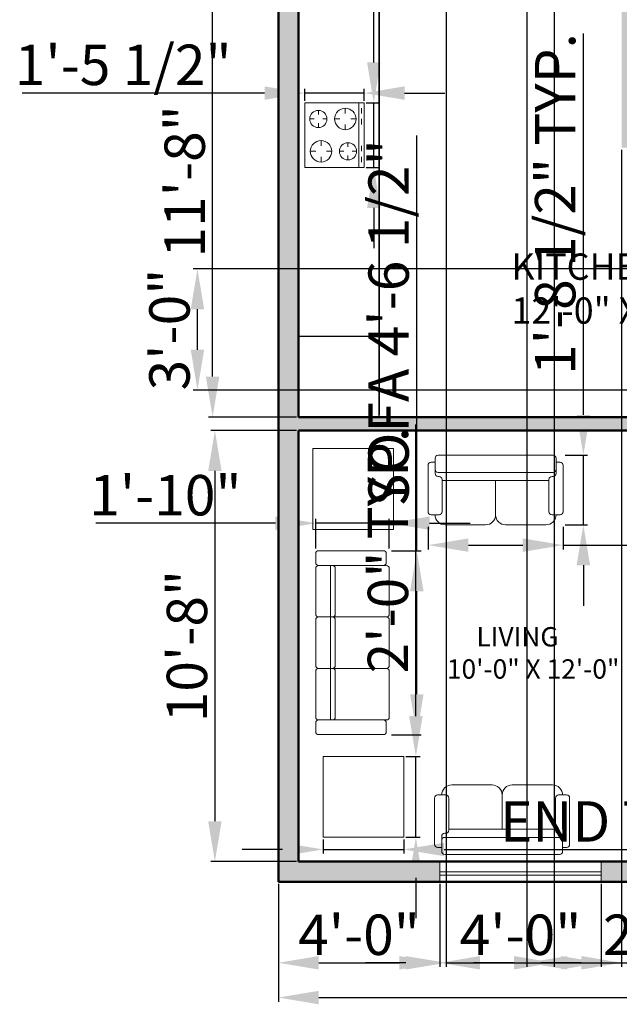
# Model space of a CAD drawing. Units: inches. Extents: x 2549 to 2991, y 1646 to 2183.
# Tile 1 of 3: x 2549 to 2727, y 1646 to 1938. Entities that reach past the tile are written whole.
import ezdxf

# ---------------------------------------------------------------- set-up
doc = ezdxf.new("R2010")
doc.units = ezdxf.units.IN
for name, color, linetype, lineweight in [('A-ANNO-DIMS', 2, 'Continuous', 18), ('A-AREA-IDEN', 7, 'Continuous', 25), ('A-EQPM', 8, 'Continuous', 20), ('A-FLOR-CASE', 8, 'Continuous', 25), ('A-FURN', 9, 'Continuous', 18), ('A-GLAZ', 4, 'Continuous', 18), ('A-WALL', 7, 'Continuous', 50)]:
    doc.layers.add(name, color=color, linetype=linetype, lineweight=lineweight)
doc.layers.add('A-WALL-PATT', color=251, linetype='Continuous', lineweight=13, true_color=0x636466)
doc.styles.get("Standard").update_dxf_attribs({"font": 'arial.ttf'})
doc.dimstyles.new('ISO-25', dxfattribs={"dimtxt": 12, "dimasz": 12, "dimexe": 1.25, "dimexo": 0.625, "dimtad": 1, "dimlunit": 3, "dimtxsty": 'Standard', "dimcen": 2.5, "dimadec": 0, "dimazin": 0, "dimtfac": 1, "dimtmove": 0, "dimatfit": 3, "dimfxl": 1, "dimarcsym": 0})

# ---------------------------------------------------------------- blocks, each defined once
blk = doc.blocks.new('A$C02A636C4')
for p, q in [((1.2026, 0.6692), (0.097, 0.6692)), ((0, 0.5722), (0, 0.1261)), ((0.0679, 0.6013), (0.0291, 0.6013)), ((0.0679, 0.6401), (0.0679, 0.6013)), ((0.0679, 0.5334), (0.0679, 0.6013)), ((1.2317, 0.6401), (1.2317, 0.6013)), ((1.2317, 0.6013), (1.2705, 0.6013)), ((1.2317, 0.5334), (1.2317, 0.6013)), ((1.2996, 0.5722), (1.2996, 0.1261)), ((0.0679, 0.4946), (0.0679, 0.5431)), ((1.2026, 0.5043), (0.097, 0.5043)), ((1.2317, 0.4946), (1.2317, 0.5431)), ((0.1067, 0.4655), (0.097, 0.4655)), ((0.1358, 0.1261), (0.1358, 0.4364)), ((1.1638, 0.4267), (0.1358, 0.4267)), ((0.6498, 0.097), (0.6498, 0.4267)), ((1.1638, 0.1261), (1.1638, 0.4364)), ((1.1929, 0.4655), (1.2026, 0.4655)), ((0.0291, 0.097), (0.1067, 0.097)), ((1.2705, 0.097), (1.1929, 0.097)), ((0.1649, 0), (0.5528, 0)), ((0.7468, 0), (1.1347, 0))]:
    blk.add_line(p, q)
for centre, radius, start, end in [((0.097, 0.6401), 0.0291, 90, 180), ((1.2026, 0.6401), 0.0291, 0, 90), ((0.0291, 0.5722), 0.0291, 90, 180), ((1.2705, 0.5722), 0.0291, 0, 90), ((0.097, 0.5334), 0.0291, 180, 270), ((0.097, 0.4946), 0.0291, 180, 270), ((1.2026, 0.5334), 0.0291, 270, 0), ((1.2026, 0.4946), 0.0291, 270, 0), ((0.1067, 0.4364), 0.0291, 0, 90), ((1.1929, 0.4364), 0.0291, 90, 180), ((0.0291, 0.1261), 0.0291, 180, 270), ((0.1649, 0.097), 0.097, 180, 270), ((0.1067, 0.1261), 0.0291, 270, 0), ((0.5528, 0.097), 0.097, 270, 0), ((0.7468, 0.097), 0.097, 180, 270), ((1.1347, 0.097), 0.097, 270, 0), ((1.1929, 0.1261), 0.0291, 180, 270), ((1.2705, 0.1261), 0.0291, 270, 0)]:
    blk.add_arc(centre, radius, start, end)
blk = doc.blocks.new('A$C0513100E')
for p, q in [((0, 0.768), (0, 0.064)), ((0.032, 0.8), (0.128, 0.8)), ((0.16, 0.768), (0.16, 0.032)), ((0.688, 0.8), (0.192, 0.8)), ((0.72, 0.768), (0.72, 0.032)), ((1.248, 0.8), (0.752, 0.8)), ((1.28, 0.768), (1.28, 0.032)), ((1.808, 0.8), (1.312, 0.8)), ((1.84, 0.032), (1.84, 0.768)), ((1.872, 0.8), (1.968, 0.8)), ((2, 0.064), (2, 0.768)), ((0.72, 0.64), (0.16, 0.64)), ((0.688, 0.587), (0.192, 0.587)), ((1.28, 0.64), (0.72, 0.64)), ((1.248, 0.587), (0.752, 0.587)), ((1.84, 0.64), (1.28, 0.64)), ((1.808, 0.587), (1.312, 0.587)), ((0.72, 0.064), (0.72, 0.402)), ((1.28, 0.064), (1.28, 0.402)), ((1.84, 0.064), (1.84, 0.402)), ((0.032, 0.032), (0.128, 0.032)), ((0.192, 0), (0.688, 0)), ((0.752, 0), (1.248, 0)), ((1.312, 0), (1.808, 0)), ((1.872, 0.032), (1.968, 0.032))]:
    blk.add_line(p, q)
for centre, start, end in [((0.032, 0.768), 90, 180), ((0.128, 0.768), 0, 90), ((0.192, 0.768), 90, 180), ((0.688, 0.768), 0, 90), ((0.752, 0.768), 90, 180), ((1.248, 0.768), 0, 90), ((1.312, 0.768), 90, 180), ((1.808, 0.768), 0, 90), ((1.872, 0.768), 90, 180), ((1.968, 0.768), 0, 90), ((0.192, 0.619), 180, 270), ((0.688, 0.619), 270, 0), ((0.752, 0.619), 180, 270), ((1.248, 0.619), 270, 0), ((1.312, 0.619), 180, 270), ((1.808, 0.619), 270, 0), ((0.032, 0.064), 180, 270), ((0.128, 0.064), 270, 0), ((0.192, 0.032), 180, 270), ((0.688, 0.032), 270, 0), ((0.752, 0.032), 180, 270), ((1.248, 0.032), 270, 0), ((1.312, 0.032), 180, 270), ((1.808, 0.032), 270, 0), ((1.872, 0.064), 180, 270), ((1.968, 0.064), 270, 0)]:
    blk.add_arc(centre, 0.032, start, end)
blk = doc.blocks.new('A$C3FB84F07')
at = {"linetype": 'ByBlock'}
for p, q in [((487.7, 447), (0, 447)), ((0, 447), (0, 0)), ((487.7, 0), (487.7, 447)), ((121.9, 406.4), (121.9, 365.8)), ((365.8, 410.5), (365.8, 378)), ((40.6, 325.1), (81.3, 325.1)), ((203.2, 325.1), (162.6, 325.1)), ((300.7, 345.4), (333.2, 345.4)), ((365.8, 280.4), (365.8, 312.9)), ((430.8, 345.4), (398.3, 345.4)), ((121.9, 243.8), (121.9, 284.5)), ((365.8, 223.5), (365.8, 182.9)), ((121.9, 186.9), (121.9, 154.4)), ((56.9, 121.9), (89.4, 121.9)), ((121.9, 56.9), (121.9, 89.4)), ((186.9, 121.9), (154.4, 121.9)), ((284.5, 142.2), (325.1, 142.2)), ((365.8, 61), (365.8, 101.6)), ((447, 142.2), (406.4, 142.2)), ((0, 40.6), (487.7, 40.6)), ((0, 0), (487.7, 0)), ((40.6, 20.3), (81.3, 20.3)), ((121.9, 20.3), (162.6, 20.3)), ((325.1, 20.3), (365.8, 20.3)), ((406.4, 20.3), (447, 20.3))]:
    blk.add_line(p, q, dxfattribs=at)
for centre, radius in [((121.9, 325.1), 81.3), ((365.8, 345.4), 65), ((365.8, 142.2), 81.3), ((121.9, 121.9), 65)]:
    blk.add_circle(centre, radius, dxfattribs=at)
blk = doc.blocks.new('*D11')
at = {"layer": 'A-ANNO-DIMS', "color": 0, "lineweight": -2, "transparency": 16777216}
for p, q in [((2631.41, 1960.26), (2605.25, 1960.26)), ((2606.5, 1832.26), (2606.5, 1948.26)), ((2631.41, 1820.26), (2605.25, 1820.26))]:
    blk.add_line(p, q, dxfattribs=at)
at = {"layer": 'A-ANNO-DIMS', "color": 0, "transparency": 16777216}
for points in [[(2604.5, 1948.26), (2608.5, 1948.26), (2606.5, 1960.26)], [(2604.5, 1832.26), (2608.5, 1832.26), (2606.5, 1820.26)]]:
    blk.add_solid(points, dxfattribs=at)
at = {"layer": 'Defpoints', "color": 0, "transparency": 16777216}
for p in [(2606.5, 1960.26), (2632.04, 1960.26), (2632.04, 1820.26)]:
    blk.add_point(p, dxfattribs=at)
at = {"layer": 'A-ANNO-DIMS', "color": 0, "transparency": 16777216, "insert": (2599.75, 1890.26), "char_height": 12, "attachment_point": 5, "rotation": 90}
blk.add_mtext('11\'-8"', dxfattribs=at)
blk = doc.blocks.new('*D12')
at = {"layer": 'A-ANNO-DIMS', "color": 0, "lineweight": -2, "transparency": 16777216}
for p, q in [((2631.41, 1816.26), (2605.92, 1816.26)), ((2607.17, 1804.26), (2607.17, 1700.26)), ((2631.41, 1688.26), (2605.92, 1688.26))]:
    blk.add_line(p, q, dxfattribs=at)
at = {"layer": 'A-ANNO-DIMS', "color": 0, "transparency": 16777216}
for points in [[(2605.17, 1804.26), (2609.17, 1804.26), (2607.17, 1816.26)], [(2605.17, 1700.26), (2609.17, 1700.26), (2607.17, 1688.26)]]:
    blk.add_solid(points, dxfattribs=at)
at = {"layer": 'Defpoints', "color": 0, "transparency": 16777216}
for p in [(2632.04, 1816.26), (2607.17, 1688.26), (2632.04, 1688.26)]:
    blk.add_point(p, dxfattribs=at)
at = {"layer": 'A-ANNO-DIMS', "color": 0, "transparency": 16777216, "insert": (2600.42, 1752.26), "char_height": 12, "attachment_point": 5, "rotation": 90}
blk.add_mtext('10\'-8"', dxfattribs=at)
blk = doc.blocks.new('*D13')
at = {"layer": 'A-ANNO-DIMS', "color": 0, "lineweight": -2, "transparency": 16777216}
for p, q in [((2626.04, 1681.64), (2626.04, 1646.63)), ((2866.04, 1681.64), (2866.04, 1646.63)), ((2638.04, 1647.88), (2854.04, 1647.88))]:
    blk.add_line(p, q, dxfattribs=at)
at = {"layer": 'A-ANNO-DIMS', "color": 0, "transparency": 16777216}
for points in [[(2638.04, 1649.88), (2638.04, 1645.88), (2626.04, 1647.88)], [(2854.04, 1649.88), (2854.04, 1645.88), (2866.04, 1647.88)]]:
    blk.add_solid(points, dxfattribs=at)
at = {"layer": 'Defpoints', "color": 0, "transparency": 16777216}
for p in [(2626.04, 1682.26), (2866.04, 1682.26), (2866.04, 1647.88)]:
    blk.add_point(p, dxfattribs=at)
at = {"layer": 'A-ANNO-DIMS', "color": 0, "transparency": 16777216, "insert": (2746.04, 1654.63), "char_height": 12, "attachment_point": 5}
blk.add_mtext("20'", dxfattribs=at)
blk = doc.blocks.new('END-TABLE-24')
for p, q in [((0, 24), (24, 24)), ((0, 0), (0, 24)), ((24, 24), (24, 0)), ((24, 0), (0, 0))]:
    blk.add_line(p, q)
blk = doc.blocks.new('*D16')
at = {"layer": 'A-ANNO-DIMS', "color": 0, "lineweight": -2, "transparency": 16777216}
for p, q in [((2670.52, 1787.63), (2670.52, 1780.98)), ((2710.65, 1787.63), (2710.65, 1780.98)), ((2682.52, 1782.23), (2698.65, 1782.23)), ((2710.65, 1782.23), (2889.68, 1782.23))]:
    blk.add_line(p, q, dxfattribs=at)
at = {"layer": 'A-ANNO-DIMS', "color": 0, "transparency": 16777216}
for points in [[(2682.52, 1784.23), (2682.52, 1780.23), (2670.52, 1782.23)], [(2698.65, 1784.23), (2698.65, 1780.23), (2710.65, 1782.23)]]:
    blk.add_solid(points, dxfattribs=at)
at = {"layer": 'Defpoints', "color": 0, "transparency": 16777216}
for p in [(2670.52, 1788.25), (2710.65, 1788.25), (2710.65, 1782.23)]:
    blk.add_point(p, dxfattribs=at)
at = {"layer": 'A-ANNO-DIMS', "color": 0, "transparency": 16777216, "insert": (2806.17, 1789.07), "char_height": 12, "attachment_point": 5}
blk.add_mtext('LOVESEAT 3\'-4" TYP.', dxfattribs=at)
blk = doc.blocks.new('*D17')
at = {"layer": 'A-ANNO-DIMS', "color": 0, "lineweight": -2, "transparency": 16777216}
for p, q in [((2716.67, 1820.92), (2716.67, 1934.15)), ((2711.28, 1808.92), (2717.92, 1808.92)), ((2716.67, 1788.25), (2716.67, 1808.92)), ((2711.28, 1788.25), (2717.92, 1788.25)), ((2716.67, 1776.25), (2716.67, 1764.25))]:
    blk.add_line(p, q, dxfattribs=at)
at = {"layer": 'A-ANNO-DIMS', "color": 0, "transparency": 16777216}
for points in [[(2714.67, 1820.92), (2718.67, 1820.92), (2716.67, 1808.92)], [(2714.67, 1776.25), (2718.67, 1776.25), (2716.67, 1788.25)]]:
    blk.add_solid(points, dxfattribs=at)
at = {"layer": 'Defpoints', "color": 0, "transparency": 16777216}
for p in [(2710.65, 1808.92), (2716.67, 1808.92), (2710.65, 1788.25)]:
    blk.add_point(p, dxfattribs=at)
at = {"layer": 'A-ANNO-DIMS', "color": 0, "transparency": 16777216, "insert": (2709.84, 1883.53), "char_height": 12, "attachment_point": 5, "rotation": 90}
blk.add_mtext('1\'-8 1/2" TYP.', dxfattribs=at)
blk = doc.blocks.new('*D18')
at = {"layer": 'A-ANNO-DIMS', "color": 0, "lineweight": -2, "transparency": 16777216}
for p, q in [((2639.3, 1694.84), (2639.3, 1690.62)), ((2663.3, 1694.84), (2663.3, 1690.62)), ((2627.3, 1691.87), (2615.3, 1691.87)), ((2639.3, 1691.87), (2663.3, 1691.87)), ((2675.3, 1691.87), (2858.88, 1691.87))]:
    blk.add_line(p, q, dxfattribs=at)
at = {"layer": 'A-ANNO-DIMS', "color": 0, "transparency": 16777216}
for points in [[(2627.3, 1693.87), (2627.3, 1689.87), (2639.3, 1691.87)], [(2675.3, 1693.87), (2675.3, 1689.87), (2663.3, 1691.87)]]:
    blk.add_solid(points, dxfattribs=at)
at = {"layer": 'Defpoints', "color": 0, "transparency": 16777216}
for p in [(2639.3, 1695.47), (2663.3, 1695.47), (2663.3, 1691.87)]:
    blk.add_point(p, dxfattribs=at)
at = {"layer": 'A-ANNO-DIMS', "color": 0, "transparency": 16777216, "insert": (2773.09, 1698.62), "char_height": 12, "attachment_point": 5}
blk.add_mtext('END TABLE 2\'-0" TYP.', dxfattribs=at)
blk = doc.blocks.new('*D19')
at = {"layer": 'A-ANNO-DIMS', "color": 0, "lineweight": -2, "transparency": 16777216}
for p, q in [((2666.9, 1731.47), (2666.9, 1818.07)), ((2663.93, 1719.47), (2668.15, 1719.47)), ((2666.9, 1695.47), (2666.9, 1719.47)), ((2663.93, 1695.47), (2668.15, 1695.47)), ((2666.9, 1683.47), (2666.9, 1671.47))]:
    blk.add_line(p, q, dxfattribs=at)
at = {"layer": 'A-ANNO-DIMS', "color": 0, "transparency": 16777216}
for points in [[(2664.9, 1731.47), (2668.9, 1731.47), (2666.9, 1719.47)], [(2664.9, 1683.47), (2668.9, 1683.47), (2666.9, 1695.47)]]:
    blk.add_solid(points, dxfattribs=at)
at = {"layer": 'Defpoints', "color": 0, "transparency": 16777216}
for p in [(2663.3, 1719.47), (2666.9, 1719.47), (2663.3, 1695.47)]:
    blk.add_point(p, dxfattribs=at)
at = {"layer": 'A-ANNO-DIMS', "color": 0, "transparency": 16777216, "insert": (2660.15, 1780.77), "char_height": 12, "attachment_point": 5, "rotation": 90}
blk.add_mtext('2\'-0" TYP.', dxfattribs=at)
blk = doc.blocks.new('*D22')
at = {"layer": 'A-ANNO-DIMS', "color": 0, "lineweight": -2, "transparency": 16777216}
for p, q in [((2667.18, 1780.56), (2667.18, 1903.91)), ((2659.61, 1780.56), (2668.43, 1780.56)), ((2667.18, 1737.95), (2667.18, 1768.56)), ((2659.61, 1725.95), (2668.43, 1725.95))]:
    blk.add_line(p, q, dxfattribs=at)
at = {"layer": 'A-ANNO-DIMS', "color": 0, "transparency": 16777216}
for points in [[(2665.18, 1768.56), (2669.18, 1768.56), (2667.18, 1780.56)], [(2665.18, 1737.95), (2669.18, 1737.95), (2667.18, 1725.95)]]:
    blk.add_solid(points, dxfattribs=at)
at = {"layer": 'Defpoints', "color": 0, "transparency": 16777216}
for p in [(2658.99, 1780.56), (2667.18, 1780.56), (2658.99, 1725.95)]:
    blk.add_point(p, dxfattribs=at)
at = {"layer": 'A-ANNO-DIMS', "color": 0, "transparency": 16777216, "insert": (2660.35, 1848.24), "char_height": 12, "attachment_point": 5, "rotation": 90}
blk.add_mtext('SOFA 4\'-6 1/2"', dxfattribs=at)
blk = doc.blocks.new('*D23')
at = {"layer": 'A-ANNO-DIMS', "color": 0, "lineweight": -2, "transparency": 16777216}
for p, q in [((2637.15, 1781.19), (2637.15, 1790)), ((2658.99, 1781.19), (2658.99, 1790)), ((2625.15, 1788.75), (2571.8, 1788.75)), ((2658.99, 1788.75), (2637.15, 1788.75)), ((2670.99, 1788.75), (2682.99, 1788.75))]:
    blk.add_line(p, q, dxfattribs=at)
at = {"layer": 'A-ANNO-DIMS', "color": 0, "transparency": 16777216}
for points in [[(2625.15, 1790.75), (2625.15, 1786.75), (2637.15, 1788.75)], [(2670.99, 1790.75), (2670.99, 1786.75), (2658.99, 1788.75)]]:
    blk.add_solid(points, dxfattribs=at)
at = {"layer": 'Defpoints', "color": 0, "transparency": 16777216}
for p in [(2637.15, 1788.75), (2637.15, 1780.56), (2658.99, 1780.56)]:
    blk.add_point(p, dxfattribs=at)
at = {"layer": 'A-ANNO-DIMS', "color": 0, "transparency": 16777216, "insert": (2592.47, 1795.5), "char_height": 12, "attachment_point": 5}
blk.add_mtext('1\'-10"', dxfattribs=at)
blk = doc.blocks.new('*D24')
at = {"layer": 'A-ANNO-DIMS', "color": 0, "lineweight": -2, "transparency": 16777216}
for p, q in [((2654.4, 1925.59), (2654.4, 2059.08)), ((2652.15, 1913.59), (2655.65, 1913.59)), ((2654.4, 1894.39), (2654.4, 1913.59)), ((2652.15, 1894.39), (2655.65, 1894.39)), ((2654.4, 1882.39), (2654.4, 1870.39))]:
    blk.add_line(p, q, dxfattribs=at)
at = {"layer": 'A-ANNO-DIMS', "color": 0, "transparency": 16777216}
for points in [[(2652.4, 1925.59), (2656.4, 1925.59), (2654.4, 1913.59)], [(2652.4, 1882.39), (2656.4, 1882.39), (2654.4, 1894.39)]]:
    blk.add_solid(points, dxfattribs=at)
at = {"layer": 'Defpoints', "color": 0, "transparency": 16777216}
for p in [(2651.52, 1913.59), (2654.4, 1913.59), (2651.52, 1894.39)]:
    blk.add_point(p, dxfattribs=at)
at = {"layer": 'A-ANNO-DIMS', "color": 0, "transparency": 16777216, "insert": (2647.57, 1998.33), "char_height": 12, "attachment_point": 5, "rotation": 90}
blk.add_mtext('COOKTOP 1\'-7"', dxfattribs=at)
blk = doc.blocks.new('*D25')
at = {"layer": 'A-ANNO-DIMS', "color": 0, "lineweight": -2, "transparency": 16777216}
for p, q in [((2621.92, 1916.47), (2549.94, 1916.47)), ((2633.92, 1914.21), (2633.92, 1917.72)), ((2651.52, 1916.47), (2633.92, 1916.47)), ((2651.52, 1914.21), (2651.52, 1917.72)), ((2663.52, 1916.47), (2675.52, 1916.47))]:
    blk.add_line(p, q, dxfattribs=at)
at = {"layer": 'A-ANNO-DIMS', "color": 0, "transparency": 16777216}
for points in [[(2621.92, 1918.47), (2621.92, 1914.47), (2633.92, 1916.47)], [(2663.52, 1918.47), (2663.52, 1914.47), (2651.52, 1916.47)]]:
    blk.add_solid(points, dxfattribs=at)
at = {"layer": 'Defpoints', "color": 0, "transparency": 16777216}
for p in [(2633.92, 1916.47), (2633.92, 1913.59), (2651.52, 1913.59)]:
    blk.add_point(p, dxfattribs=at)
at = {"layer": 'A-ANNO-DIMS', "color": 0, "transparency": 16777216, "insert": (2579.93, 1923.3), "char_height": 12, "attachment_point": 5}
blk.add_mtext('1\'-5 1/2"', dxfattribs=at)
blk = doc.blocks.new('*D28')
at = {"layer": 'A-ANNO-DIMS', "color": 0, "lineweight": -2, "transparency": 16777216}
for p, q in [((2673.99, 1681.64), (2673.99, 1656.96)), ((2721.99, 1681.64), (2721.99, 1656.96)), ((2685.99, 1658.21), (2709.99, 1658.21))]:
    blk.add_line(p, q, dxfattribs=at)
at = {"layer": 'A-ANNO-DIMS', "color": 0, "transparency": 16777216}
for points in [[(2685.99, 1660.21), (2685.99, 1656.21), (2673.99, 1658.21)], [(2709.99, 1660.21), (2709.99, 1656.21), (2721.99, 1658.21)]]:
    blk.add_solid(points, dxfattribs=at)
at = {"layer": 'Defpoints', "color": 0, "transparency": 16777216}
for p in [(2673.99, 1682.26), (2721.99, 1682.26), (2721.99, 1658.21)]:
    blk.add_point(p, dxfattribs=at)
at = {"layer": 'A-ANNO-DIMS', "color": 0, "transparency": 16777216, "insert": (2697.99, 1664.97), "char_height": 12, "attachment_point": 5}
blk.add_mtext('4\'-0"', dxfattribs=at)
blk = doc.blocks.new('*D29')
at = {"layer": 'A-ANNO-DIMS', "color": 0, "lineweight": -2, "transparency": 16777216}
for p, q in [((2626.04, 1681.64), (2626.04, 1656.96)), ((2673.99, 1681.64), (2673.99, 1656.96)), ((2638.04, 1658.21), (2661.99, 1658.21))]:
    blk.add_line(p, q, dxfattribs=at)
at = {"layer": 'A-ANNO-DIMS', "color": 0, "transparency": 16777216}
for points in [[(2638.04, 1660.21), (2638.04, 1656.21), (2626.04, 1658.21)], [(2661.99, 1660.21), (2661.99, 1656.21), (2673.99, 1658.21)]]:
    blk.add_solid(points, dxfattribs=at)
at = {"layer": 'Defpoints', "color": 0, "transparency": 16777216}
for p in [(2626.04, 1682.26), (2673.99, 1682.26), (2673.99, 1658.21)]:
    blk.add_point(p, dxfattribs=at)
at = {"layer": 'A-ANNO-DIMS', "color": 0, "transparency": 16777216, "insert": (2650.01, 1664.97), "char_height": 12, "attachment_point": 5}
blk.add_mtext('4\'-0"', dxfattribs=at)
blk = doc.blocks.new('*D33')
at = {"layer": 'A-ANNO-DIMS', "color": 0, "lineweight": -2, "transparency": 16777216}
for p, q in [((2675.89, 1963.64), (2675.89, 1656.96)), ((2699.89, 1963.64), (2699.89, 1656.96)), ((2663.89, 1658.21), (2651.89, 1658.21)), ((2675.89, 1658.21), (2699.89, 1658.21)), ((2711.89, 1658.21), (2757.24, 1658.21))]:
    blk.add_line(p, q, dxfattribs=at)
at = {"layer": 'A-ANNO-DIMS', "color": 0, "transparency": 16777216}
for points in [[(2663.89, 1660.21), (2663.89, 1656.21), (2675.89, 1658.21)], [(2711.89, 1660.21), (2711.89, 1656.21), (2699.89, 1658.21)]]:
    blk.add_solid(points, dxfattribs=at)
at = {"layer": 'Defpoints', "color": 0, "transparency": 16777216}
for p in [(2675.89, 1964.26), (2699.89, 1964.26), (2699.89, 1658.21)]:
    blk.add_point(p, dxfattribs=at)
at = {"layer": 'A-ANNO-DIMS', "color": 0, "transparency": 16777216, "insert": (2740.57, 1664.97), "char_height": 12, "attachment_point": 5}
blk.add_mtext('2\'-0"', dxfattribs=at)
blk = doc.blocks.new('*D40')
at = {"layer": 'A-ANNO-DIMS', "color": 0, "lineweight": -2, "transparency": 16777216}
for p, q in [((2799.41, 1864.26), (2600.74, 1864.26)), ((2601.99, 1840.26), (2601.99, 1852.26)), ((2799.41, 1828.26), (2600.74, 1828.26))]:
    blk.add_line(p, q, dxfattribs=at)
at = {"layer": 'A-ANNO-DIMS', "color": 0, "transparency": 16777216}
for points in [[(2599.99, 1852.26), (2603.99, 1852.26), (2601.99, 1864.26)], [(2599.99, 1840.26), (2603.99, 1840.26), (2601.99, 1828.26)]]:
    blk.add_solid(points, dxfattribs=at)
at = {"layer": 'Defpoints', "color": 0, "transparency": 16777216}
for p in [(2601.99, 1864.26), (2800.04, 1864.26), (2800.04, 1828.26)]:
    blk.add_point(p, dxfattribs=at)
at = {"layer": 'A-ANNO-DIMS', "color": 0, "transparency": 16777216, "insert": (2595.23, 1846.26), "char_height": 12, "attachment_point": 5, "rotation": 90}
blk.add_mtext('3\'-0"', dxfattribs=at)
blk = doc.blocks.new('*D41')
at = {"layer": 'A-ANNO-DIMS', "color": 0, "lineweight": -2, "transparency": 16777216}
for p, q in [((2632.04, 1820.89), (2632.04, 2067.56)), ((2656.04, 1820.89), (2656.04, 2067.56)), ((2620.04, 2066.31), (2608.04, 2066.31)), ((2632.04, 2066.31), (2656.04, 2066.31)), ((2668.04, 2066.31), (2713.39, 2066.31))]:
    blk.add_line(p, q, dxfattribs=at)
at = {"layer": 'A-ANNO-DIMS', "color": 0, "transparency": 16777216}
for points in [[(2620.04, 2068.31), (2620.04, 2064.31), (2632.04, 2066.31)], [(2668.04, 2068.31), (2668.04, 2064.31), (2656.04, 2066.31)]]:
    blk.add_solid(points, dxfattribs=at)
at = {"layer": 'Defpoints', "color": 0, "transparency": 16777216}
for p in [(2656.04, 2066.31), (2632.04, 1820.26), (2656.04, 1820.26)]:
    blk.add_point(p, dxfattribs=at)
at = {"layer": 'A-ANNO-DIMS', "color": 0, "transparency": 16777216, "insert": (2696.72, 2073.07), "char_height": 12, "attachment_point": 5}
blk.add_mtext('2\'-0"', dxfattribs=at)
blk = doc.blocks.new('*D44')
at = {"layer": 'A-ANNO-DIMS', "color": 0, "lineweight": -2, "transparency": 16777216}
for p, q in [((2708.04, 1963.64), (2708.04, 1656.96)), ((2732.04, 1963.64), (2732.04, 1656.96)), ((2696.04, 1658.21), (2684.04, 1658.21)), ((2708.04, 1658.21), (2732.04, 1658.21)), ((2744.04, 1658.21), (2789.39, 1658.21))]:
    blk.add_line(p, q, dxfattribs=at)
at = {"layer": 'A-ANNO-DIMS', "color": 0, "transparency": 16777216}
for points in [[(2696.04, 1660.21), (2696.04, 1656.21), (2708.04, 1658.21)], [(2744.04, 1660.21), (2744.04, 1656.21), (2732.04, 1658.21)]]:
    blk.add_solid(points, dxfattribs=at)
at = {"layer": 'Defpoints', "color": 0, "transparency": 16777216}
for p in [(2708.04, 1964.26), (2732.04, 1964.26), (2732.04, 1658.21)]:
    blk.add_point(p, dxfattribs=at)
at = {"layer": 'A-ANNO-DIMS', "color": 0, "transparency": 16777216, "insert": (2772.72, 1664.97), "char_height": 12, "attachment_point": 5}
blk.add_mtext('2\'-0"', dxfattribs=at)
blk = doc.blocks.new('*D49')
at = {"layer": 'A-ANNO-DIMS', "color": 0, "lineweight": -2, "transparency": 16777216}
for p, q in [((2732.04, 1903.64), (2732.04, 1656.96)), ((2728.04, 1899.64), (2728.04, 1656.96)), ((2716.04, 1658.21), (2704.04, 1658.21)), ((2728.04, 1658.21), (2732.04, 1658.21)), ((2744.04, 1658.21), (2789.19, 1658.21))]:
    blk.add_line(p, q, dxfattribs=at)
at = {"layer": 'A-ANNO-DIMS', "color": 0, "transparency": 16777216}
for points in [[(2716.04, 1660.21), (2716.04, 1656.21), (2728.04, 1658.21)], [(2744.04, 1660.21), (2744.04, 1656.21), (2732.04, 1658.21)]]:
    blk.add_solid(points, dxfattribs=at)
at = {"layer": 'Defpoints', "color": 0, "transparency": 16777216}
for p in [(2732.04, 1904.26), (2728.04, 1900.26), (2732.04, 1658.21)]:
    blk.add_point(p, dxfattribs=at)
at = {"layer": 'A-ANNO-DIMS', "color": 0, "transparency": 16777216, "insert": (2772.61, 1664.97), "char_height": 12, "attachment_point": 5}
blk.add_mtext('0\'-4"', dxfattribs=at)

msp = doc.modelspace()

# ---------------------------------------------------------------- hatches: boundary and pattern name
at = {"layer": 'A-WALL-PATT'}
h = msp.add_hatch(color=256, dxfattribs=at)
h.dxf.hatch_style = 1
h.paths.add_polyline_path([(2765.46, 2042.264), (2626.038, 2042.264), (2626.038, 1682.264), (2673.991, 1682.264), (2673.991, 1688.264), (2632.038, 1688.264), (2632.038, 1816.264), (2752.038, 1816.264), (2752.038, 1811.649), (2756.038, 1811.649), (2756.038, 1820.264), (2632.038, 1820.264), (2632.038, 1960.264), (2675.89, 1960.264), (2675.89, 1964.264), (2632.038, 1964.264), (2632.038, 2036.264), (2704.038, 2036.264), (2704.038, 1964.264), (2699.89, 1964.264), (2699.89, 1960.264), (2728.038, 1960.264), (2728.038, 1900.264), (2734.981, 1900.264), (2734.981, 1904.264), (2732.038, 1904.264), (2732.038, 1964.264), (2708.038, 1964.264), (2708.038, 2036.264), (2765.46, 2036.264)])
h.paths.add_polyline_path([(2866.038, 2042.264), (2825.46, 2042.264), (2825.46, 2036.264), (2860.038, 2036.264), (2860.038, 1904.264), (2770.981, 1904.264), (2770.981, 1900.264), (2860.038, 1900.264), (2860.038, 1688.264), (2852.256, 1688.264), (2852.256, 1682.264), (2866.038, 1682.264)])
h.paths.add_polyline_path([(2816.256, 1688.264), (2756.038, 1688.264), (2756.038, 1775.649), (2752.038, 1775.649), (2752.038, 1688.264), (2721.991, 1688.264), (2721.991, 1682.264), (2816.256, 1682.264)])

# ---------------------------------------------------------------- linework, layer by layer
at = {"layer": 'A-FLOR-CASE'}
for p, q in [((2656.038, 1820.264), (2656.038, 1960.264)), ((2632.038, 1844.264), (2656.038, 1844.264))]:
    msp.add_line(p, q, dxfattribs=at)
at = {"layer": 'A-GLAZ'}
for p, q in [((2673.991, 1688.264), (2673.991, 1682.264)), ((2721.991, 1688.264), (2721.991, 1682.264)), ((2721.991, 1685.264), (2673.991, 1685.264)), ((2721.991, 1684.264), (2673.991, 1684.264))]:
    msp.add_line(p, q, dxfattribs=at)
at = {"layer": 'A-WALL'}
for p, q in [((2626.038, 1682.264), (2626.038, 2042.264)), ((2632.038, 1820.264), (2632.038, 1960.264)), ((2632.038, 1820.264), (2756.038, 1820.264)), ((2632.038, 1688.264), (2632.038, 1816.264)), ((2632.038, 1816.264), (2752.038, 1816.264)), ((2752.038, 1688.264), (2632.038, 1688.264)), ((2816.256, 1682.264), (2626.038, 1682.264))]:
    msp.add_line(p, q, dxfattribs=at)

# ---------------------------------------------------------------- block references
at = {"layer": 'A-EQPM', "xscale": 0.0393700787401575, "yscale": 0.0393700787401575, "zscale": 0.0393700787401575, "rotation": 90}
msp.add_blockref('A$C3FB84F07', (2651.523, 1894.387), dxfattribs=at)
at = {"layer": 'A-FURN'}
for p in [(2636.293, 1786.903), (2639.3, 1695.469)]:
    msp.add_blockref('END-TABLE-24', p, dxfattribs=at)
at = {"layer": 'A-FURN', "xscale": 30.88031007495567, "yscale": 30.88031007495567, "zscale": 30.88031007495567}
msp.add_blockref('A$C02A636C4', (2670.518, 1788.253), dxfattribs=at)
at = {"layer": 'A-FURN'}
for name, p, xscale, yscale, zscale, rotation in [('A$C0513100E', (2658.988, 1725.955), 27.30306626343093, 27.30306626343093, 27.30306626343093, 90), ('A$C02A636C4', (2712.599, 1711.033), 30.88031007495567, 30.88031007495567, 30.88031007495567, 180.0000000000145)]:
    msp.add_blockref(name, p, dxfattribs=dict(at, xscale=xscale, yscale=yscale, zscale=zscale, rotation=rotation))

# ---------------------------------------------------------------- texts
at = {"layer": 'A-AREA-IDEN', "attachment_point": 1}
for s, width, gutter_width, insert, char_height in [('KITCHEN / DINING\\P12\'-0" X 14\'-0"', 272.27661, 39.11, (2695.29, 1868.84), 7.82199), ('     LIVING\\P10\'-0" X 12\'-0"', 199.71745, 28.687, (2676.124, 1757.89), 5.7375)]:
    msp.add_mtext_dynamic_manual_height_columns(s, width=width, gutter_width=gutter_width, heights=[0], dxfattribs=dict(at, insert=insert, char_height=char_height))

# ---------------------------------------------------------------- dimensions: what is measured, and where the dimension line sits
at = {"layer": 'A-ANNO-DIMS'}
for base, p1, p2, override, picture, middle in [((2656.038, 2066.314), (2632.038, 1820.264), (2656.038, 1820.264), {"dimdec": 1, "dimlfac": 1, "dimrnd": 0, "dimzin": 1, "dimdsep": 46, "dimlunit": 4, "dimfrac": 2}, '*D41', (2696.715, 2073.066)), ((2699.89, 1658.214), (2675.89, 1964.264), (2699.89, 1964.264), {"dimdec": 1, "dimlfac": 1, "dimrnd": 0, "dimzin": 1, "dimdsep": 46, "dimlunit": 4, "dimfrac": 2}, '*D33', (2740.567, 1664.966)), ((2732.038, 1658.214), (2708.038, 1964.264), (2732.038, 1964.264), {"dimdec": 1, "dimlfac": 1, "dimrnd": 0, "dimzin": 1, "dimdsep": 46, "dimlunit": 4, "dimfrac": 2}, '*D44', (2772.715, 1664.966)), ((2732.038, 1658.214), (2728.038, 1900.264), (2732.038, 1904.264), {"dimdec": 1, "dimlfac": 1, "dimrnd": 0, "dimzin": 1, "dimdsep": 46, "dimlunit": 4, "dimfrac": 2}, '*D49', (2772.613, 1664.966)), ((2866.038, 1647.88), (2626.038, 1682.264), (2866.038, 1682.264), {"dimclrd": 0, "dimclre": 0, "dimclrt": 0}, '*D13', (2746.038, 1654.632)), ((2673.991, 1658.214), (2626.038, 1682.264), (2673.991, 1682.264), {"dimdec": 1, "dimlfac": 1, "dimrnd": 0, "dimzin": 1, "dimdsep": 46, "dimlunit": 4, "dimfrac": 2}, '*D29', (2650.014, 1664.966)), ((2721.991, 1658.214), (2673.991, 1682.264), (2721.991, 1682.264), {"dimdec": 1, "dimlfac": 1, "dimrnd": 0, "dimzin": 1, "dimdsep": 46, "dimlunit": 4, "dimfrac": 2}, '*D28', (2697.991, 1664.966))]:
    dim = msp.add_linear_dim(base=base, p1=p1, p2=p2, dimstyle='ISO-25', override=override, dxfattribs=at)
    dim.commit()
    dim.dimension.update_dxf_attribs({"geometry": picture, "text_midpoint": middle})
for base, p1, p2, text, picture, middle in [((2654.403, 1913.587), (2651.523, 1894.387), (2651.523, 1913.587), 'COOKTOP <>', '*D24', (2647.569, 1998.335)), ((2716.671, 1808.918), (2710.651, 1788.253), (2710.651, 1808.918), '<> TYP.', '*D17', (2709.841, 1883.532)), ((2667.179, 1780.561), (2658.988, 1725.955), (2658.988, 1780.561), 'SOFA <>', '*D22', (2660.345, 1848.238)), ((2666.9, 1719.469), (2663.3, 1695.469), (2663.3, 1719.469), '<> TYP.', '*D19', (2660.149, 1780.769))]:
    dim = msp.add_linear_dim(base=base, p1=p1, p2=p2, angle=90, text=text, dimstyle='ISO-25', override={"dimdec": 1, "dimlfac": 1, "dimrnd": 0, "dimzin": 1, "dimdsep": 46, "dimlunit": 4, "dimfrac": 2}, dxfattribs=at)
    dim.commit()
    dim.dimension.update_dxf_attribs({"geometry": picture, "text_midpoint": middle})
for base, p1, p2, angle, override, picture, middle in [((2606.503, 1960.264), (2632.038, 1820.264), (2632.038, 1960.264), 90, {"dimclrd": 0, "dimclre": 0, "dimclrt": 0}, '*D11', (2599.751, 1890.264)), ((2633.923, 1916.467), (2651.523, 1913.587), (2633.923, 1913.587), 180, {"dimdec": 1, "dimlfac": 1, "dimrnd": 0, "dimzin": 1, "dimdsep": 46, "dimlunit": 4, "dimfrac": 2}, '*D25', (2579.932, 1923.297)), ((2601.988, 1864.264), (2800.038, 1828.264), (2800.038, 1864.264), 90, {"dimdec": 1, "dimlfac": 1, "dimrnd": 0, "dimzin": 1, "dimdsep": 46, "dimlunit": 4, "dimfrac": 2}, '*D40', (2595.232, 1846.264)), ((2607.173, 1688.264), (2632.038, 1816.264), (2632.038, 1688.264), 90, {"dimclrd": 0, "dimclre": 0, "dimclrt": 0}, '*D12', (2600.421, 1752.264)), ((2637.146, 1788.752), (2658.988, 1780.561), (2637.146, 1780.561), 180, {"dimdec": 1, "dimlfac": 1, "dimrnd": 0, "dimzin": 1, "dimdsep": 46, "dimlunit": 4, "dimfrac": 2}, '*D23', (2592.474, 1795.504))]:
    dim = msp.add_linear_dim(base=base, p1=p1, p2=p2, angle=angle, dimstyle='ISO-25', override=override, dxfattribs=at)
    dim.commit()
    dim.dimension.update_dxf_attribs({"geometry": picture, "text_midpoint": middle})
for base, p1, p2, text, picture, middle in [((2710.651, 1782.233), (2670.518, 1788.253), (2710.651, 1788.253), 'LOVESEAT <> TYP.', '*D16', (2806.167, 1789.071)), ((2663.3, 1691.869), (2639.3, 1695.469), (2663.3, 1695.469), 'END TABLE <> TYP.', '*D18', (2773.092, 1698.62))]:
    dim = msp.add_linear_dim(base=base, p1=p1, p2=p2, text=text, dimstyle='ISO-25', override={"dimdec": 1, "dimlfac": 1, "dimrnd": 0, "dimzin": 1, "dimdsep": 46, "dimlunit": 4, "dimfrac": 2}, dxfattribs=at)
    dim.commit()
    dim.dimension.update_dxf_attribs({"geometry": picture, "text_midpoint": middle})

doc.saveas('drawing.dxf')
